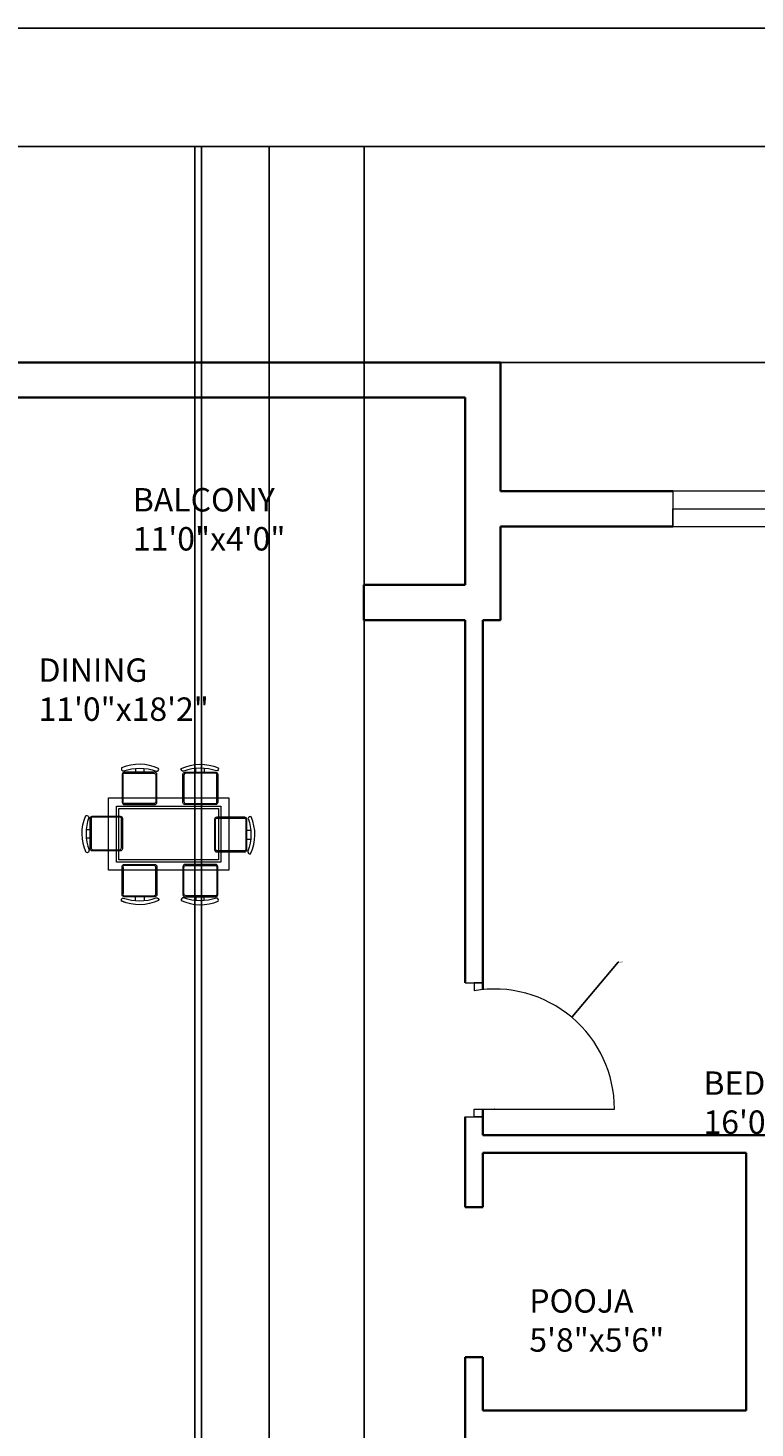
# Model space of a CAD drawing. Units: inches. Extents: x 1902 to 2626, y 1199 to 2408.
# Tile 8 of 9: x 2220 to 2407, y 2049 to 2408. Entities that reach past the tile are written whole.
import ezdxf

# ---------------------------------------------------------------- set-up
doc = ezdxf.new("R2010")
doc.units = ezdxf.units.IN
for name, color, linetype, lineweight in [('A-ANNO-DIMS', 2, 'Continuous', 18), ('A-ANNO-TTLB', 7, 'Continuous', 25), ('A-AREA-IDEN', 7, 'Continuous', 18), ('A-DOOR', 31, 'Continuous', 18), ('A-FURN', 8, 'Continuous', 13), ('A-GLAZ', 181, 'Continuous', 18), ('A-WALL', 7, 'Continuous', 35)]:
    doc.layers.add(name, color=color, linetype=linetype, lineweight=lineweight)
doc.styles.get("Standard").update_dxf_attribs({"font": 'arial.ttf'})
doc.dimstyles.get("Standard").update_dxf_attribs({"dimtxt": 0.18, "dimasz": 0.18, "dimexe": 0.18, "dimexo": 0.0625, "dimgap": 0.09, "dimtad": 0, "dimtih": 1, "dimtoh": 1, "dimdec": 4, "dimzin": 0, "dimdsep": 46, "dimtxsty": 'Standard', "dimcen": 0.09, "dimadec": 0, "dimazin": 0, "dimtfac": 1, "dimtdec": 4, "dimtofl": 0, "dimtmove": 0, "dimatfit": 3, "dimfxl": 1, "dimtolj": 1, "dimtzin": 0, "dimarcsym": 0})

# ---------------------------------------------------------------- blocks, each defined once
blk = doc.blocks.new('WINDOW-60-A')
for p, q in [((0, 9), (0, 0)), ((60, 9), (0, 9)), ((60, 4.5), (60, 9)), ((60, 9), (60, 0)), ((0, 0), (0, 4.5)), ((0, 4.5), (60, 4.5)), ((0, 0), (60, 0))]:
    blk.add_line(p, q)
blk = doc.blocks.new('TABLE-DINING-RECT')
for points in [[(0, 18.51), (30.84, 18.51), (30.84, 0), (0, 0)], [(2.06, 16.45), (28.79, 16.45), (28.79, 2.06), (2.06, 2.06)], [(2.67, 15.83), (28.17, 15.83), (28.17, 2.67), (2.67, 2.67)]]:
    blk.add_lwpolyline(points, close=True)
blk = doc.blocks.new('CHAIR-DINING')
for points in [[(8.55, 2.06), (0.75, 2.06, -0.414214), (0.2, 2.6), (0.2, 9.77, -0.414214), (0.75, 10.32), (8.55, 10.32, -0.414214), (9.09, 9.77), (9.09, 2.6, -0.414214), (8.55, 2.06)], [(8.91, 1.78, -0.578392), (9.54, 1.08, -0.214524), (0.06, 0.96, -0.552014), (0.5, 1.72, 0.175809), (8.91, 1.78)], [(5.81, 2.06), (5.81, 1.07, 0.064759)]]:
    blk.add_lwpolyline(points, format="xyb")
blk.add_lwpolyline([(0.75, 2.3), (8.3, 2.3, 0.414214), (8.85, 2.85), (8.85, 9.53, 0.414214), (8.3, 10.07), (0.75, 10.07, 0.512069), (0.45, 9.53), (0.45, 2.85, 0.512069)], format="xyb", close=True)
blk.add_lwpolyline([(3.63, 1.05), (3.63, 2.06)])
blk = doc.blocks.new('*D28')
at = {"layer": 'A-ANNO-DIMS', "color": 0, "lineweight": -2, "transparency": 16777216}
for p, q in [((1999.35, 2289.54), (1999.35, 2377.95)), ((1999.53, 2377.77), (2268.21, 2377.77)), ((2537.67, 2377.77), (2269, 2377.77)), ((2537.85, 2289.54), (2537.85, 2377.95))]:
    blk.add_line(p, q, dxfattribs=at)
at = {"layer": 'A-ANNO-DIMS', "color": 0, "transparency": 16777216}
for points in [[(1999.53, 2377.8), (1999.53, 2377.74), (1999.35, 2377.77)], [(2537.67, 2377.8), (2537.67, 2377.74), (2537.85, 2377.77)]]:
    blk.add_solid(points, dxfattribs=at)
at = {"layer": 'Defpoints', "color": 0, "transparency": 16777216}
for p in [(2537.85, 2377.77), (1999.35, 2289.47), (2537.85, 2289.47)]:
    blk.add_point(p, dxfattribs=at)
at = {"layer": 'A-ANNO-DIMS', "color": 0, "transparency": 16777216, "insert": (2268.6, 2377.77), "char_height": 0.18, "attachment_point": 5}
blk.add_mtext('\\A1;538.5', dxfattribs=at)
blk = doc.blocks.new('*D35')
at = {"layer": 'A-ANNO-DIMS', "color": 0, "lineweight": -2, "transparency": 16777216}
for p, q in [((2341.41, 2322.47), (2593.33, 2322.47)), ((2593.15, 2322.29), (2593.15, 2306.16)), ((2593.15, 2289.65), (2593.15, 2305.79)), ((2537.91, 2289.47), (2593.33, 2289.47))]:
    blk.add_line(p, q, dxfattribs=at)
at = {"layer": 'A-ANNO-DIMS', "color": 0, "transparency": 16777216}
for points in [[(2593.12, 2322.29), (2593.18, 2322.29), (2593.15, 2322.47)], [(2593.12, 2289.65), (2593.18, 2289.65), (2593.15, 2289.47)]]:
    blk.add_solid(points, dxfattribs=at)
at = {"layer": 'Defpoints', "color": 0, "transparency": 16777216}
for p in [(2341.35, 2322.47), (2593.15, 2322.47), (2537.85, 2289.47)]:
    blk.add_point(p, dxfattribs=at)
at = {"layer": 'A-ANNO-DIMS', "color": 0, "transparency": 16777216, "insert": (2593.15, 2305.97), "char_height": 0.18, "attachment_point": 5}
blk.add_mtext('\\A1;33', dxfattribs=at)
blk = doc.blocks.new('*D41')
at = {"layer": 'A-ANNO-DIMS', "color": 0, "lineweight": -2, "transparency": 16777216}
for p, q in [((2264.77, 1723.47), (2264.77, 2377.95)), ((2264.95, 2377.77), (2285.22, 2377.77)), ((2306.27, 2377.77), (2286.01, 2377.77)), ((2306.45, 1723.47), (2306.45, 2377.95))]:
    blk.add_line(p, q, dxfattribs=at)
at = {"layer": 'A-ANNO-DIMS', "color": 0, "transparency": 16777216}
for points in [[(2264.95, 2377.8), (2264.95, 2377.74), (2264.77, 2377.77)], [(2306.27, 2377.8), (2306.27, 2377.74), (2306.45, 2377.77)]]:
    blk.add_solid(points, dxfattribs=at)
at = {"layer": 'Defpoints', "color": 0, "transparency": 16777216}
for p in [(2306.45, 2377.77), (2264.77, 1723.41), (2306.45, 1723.41)]:
    blk.add_point(p, dxfattribs=at)
at = {"layer": 'A-ANNO-DIMS', "color": 0, "transparency": 16777216, "insert": (2285.61, 2377.77), "char_height": 0.18, "attachment_point": 5}
blk.add_mtext('\\A1;41.68', dxfattribs=at)
blk = doc.blocks.new('*D43')
at = {"layer": 'A-ANNO-DIMS', "color": 0, "lineweight": -2, "transparency": 16777216}
for p, q in [((2263.07, 1800.47), (2263.07, 2377.95)), ((2263.25, 2377.77), (2272.13, 2377.77)), ((2281.92, 2377.77), (2273.04, 2377.77)), ((2282.1, 1800.47), (2282.1, 2377.95))]:
    blk.add_line(p, q, dxfattribs=at)
at = {"layer": 'A-ANNO-DIMS', "color": 0, "transparency": 16777216}
for points in [[(2263.25, 2377.8), (2263.25, 2377.74), (2263.07, 2377.77)], [(2281.92, 2377.8), (2281.92, 2377.74), (2282.1, 2377.77)]]:
    blk.add_solid(points, dxfattribs=at)
at = {"layer": 'Defpoints', "color": 0, "transparency": 16777216}
for p in [(2282.1, 2377.77), (2263.07, 1800.41), (2282.1, 1800.41)]:
    blk.add_point(p, dxfattribs=at)
at = {"layer": 'A-ANNO-DIMS', "color": 0, "transparency": 16777216, "insert": (2272.58, 2377.77), "char_height": 0.18, "attachment_point": 5}
blk.add_mtext('\\A1;19.024', dxfattribs=at)
blk = doc.blocks.new('*D46')
at = {"layer": 'A-ANNO-DIMS', "color": 0, "lineweight": -2, "transparency": 16777216}
for p, q in [((2371.55, 2168.82), (2359.77, 2154.83)), ((2371.73, 2168.82), (2371.55, 2168.82)), ((2339.74, 2131.16), (2339.92, 2131.16)), ((2339.83, 2131.07), (2339.83, 2131.25))]:
    blk.add_line(p, q, dxfattribs=at)
at = {"layer": 'A-ANNO-DIMS', "color": 0, "transparency": 16777216}
blk.add_solid([(2359.75, 2154.85), (2359.79, 2154.81), (2359.65, 2154.7)], dxfattribs=at)
at = {"layer": 'Defpoints', "color": 0, "transparency": 16777216}
for p in [(2359.65, 2154.7), (2339.83, 2131.16)]:
    blk.add_point(p, dxfattribs=at)
at = {"layer": 'A-ANNO-DIMS', "color": 0, "transparency": 16777216, "insert": (2372.28, 2168.82), "char_height": 0.18, "attachment_point": 5}
blk.add_mtext('\\A1;R30.775', dxfattribs=at)

msp = doc.modelspace()

# ---------------------------------------------------------------- linework, layer by layer
at = {"layer": 'A-ANNO-TTLB'}
msp.add_lwpolyline([(1901.6928, 2408.1473), (2626.1646, 2408.1473), (2626.1646, 1206.3103), (1901.6928, 1206.3103)], close=True, dxfattribs=at)
at = {"layer": 'A-DOOR'}
for p, q in [((2332.3507, 2163.4878), (2336.8507, 2163.4878)), ((2336.8507, 2163.4878), (2334.6007, 2163.4878)), ((2334.6007, 2163.4878), (2334.6007, 2161.4878)), ((2334.6007, 2129.1591), (2334.6007, 2131.1591)), ((2334.6007, 2131.1591), (2370.6007, 2131.1591)), ((2332.3507, 2129.1591), (2336.8507, 2129.1591)), ((2336.8507, 2129.1591), (2334.6007, 2129.1591))]:
    msp.add_line(p, q, dxfattribs=at)
msp.add_arc((2339.8252, 2131.1591), 30.7755, 360, 99.774014, dxfattribs=at)
at = {"layer": 'A-FURN'}
for points in [[(2244.7449, 2217.8014, -0.17580919), (2253.1458, 2217.7377, 0.57839206), (2253.7822, 2218.4376, 0.21452438), (2244.2994, 2218.5648, 0.55201397), (2244.7449, 2217.8014, -0.06507904)], [(2244.7449, 2217.801, -0.17580919), (2253.1458, 2217.7374, 0.57839206), (2253.7822, 2218.4372, 0.21452438), (2244.2994, 2218.5645, 0.55201397), (2244.7449, 2217.801, -0.06507904)], [(2252.7893, 2217.4642), (2244.9903, 2217.4642, 0.41421356), (2244.4446, 2216.9186), (2244.4446, 2209.7475, 0.41421356), (2244.9903, 2209.2018), (2252.7893, 2209.2018, 0.41421356), (2253.335, 2209.7475), (2253.335, 2216.9186, 0.41421356), (2252.7893, 2217.4642)], [(2252.7894, 2217.4639), (2244.9903, 2217.4639, 0.41421356), (2244.4447, 2216.9182), (2244.4447, 2209.7471, 0.41421356), (2244.9903, 2209.2015), (2252.7894, 2209.2015, 0.41421356), (2253.335, 2209.7471), (2253.335, 2216.9182, 0.41421356), (2252.7894, 2217.4639)], [(2250.0499, 2217.4642), (2250.0499, 2218.4505, -0.06475861)], [(2250.0499, 2217.4639), (2250.0499, 2218.4502, -0.06475861)], [(2260.2182, 2217.7377, -0.57839206), (2259.5818, 2218.4376, -0.21452438), (2269.0645, 2218.5648, -0.55201397), (2268.619, 2217.8014, 0.1758092), (2260.2182, 2217.7378)], [(2260.2182, 2217.7374, -0.57839206), (2259.5818, 2218.4372, -0.21452438), (2269.0646, 2218.5645, -0.55201397), (2268.6191, 2217.801, 0.1758092), (2260.2182, 2217.7374)], [(2268.3737, 2217.4642, -0.41421356), (2268.9193, 2216.9186), (2268.9193, 2209.7475, -0.41421356), (2268.3737, 2209.2018), (2260.5746, 2209.2018, -0.41421356), (2260.029, 2209.7475), (2260.029, 2216.9186, -0.41421356), (2260.5746, 2217.4642), (2268.3737, 2217.4642)], [(2268.3737, 2217.4639, -0.41421356), (2268.9193, 2216.9182), (2268.9193, 2209.7471, -0.41421356), (2268.3737, 2209.2015), (2260.5746, 2209.2015, -0.41421356), (2260.029, 2209.7471), (2260.029, 2216.9182, -0.41421356), (2260.5746, 2217.4639), (2268.3737, 2217.4639)], [(2263.314, 2217.4642), (2263.314, 2218.4505, 0.06475861)], [(2263.314, 2217.4639), (2263.314, 2218.4502, 0.06475861)], [(2235.956, 2197.5146, -0.57839206), (2235.2562, 2196.8782, -0.21452438), (2235.129, 2206.3609, -0.55201397), (2235.8924, 2205.9154, 0.17580937), (2235.956, 2197.5146)], [(2235.956, 2197.5143, -0.57839206), (2235.2562, 2196.8778, -0.21452438), (2235.129, 2206.3606, -0.55201397), (2235.8924, 2205.9151, 0.17580937), (2235.956, 2197.5143)], [(2236.2296, 2205.6701, -0.41421356), (2236.7752, 2206.2157), (2243.9463, 2206.2157, -0.41421356), (2244.4919, 2205.6701), (2244.4919, 2197.871, -0.41421356), (2243.9463, 2197.3254), (2236.7752, 2197.3254, -0.41421356), (2236.2296, 2197.871), (2236.2296, 2205.6701)], [(2236.2296, 2205.6697, -0.41421356), (2236.7752, 2206.2154), (2243.9463, 2206.2154, -0.41421356), (2244.4919, 2205.6697), (2244.4919, 2197.8707, -0.41421356), (2243.9463, 2197.325), (2236.7752, 2197.325, -0.41421356), (2236.2296, 2197.8707), (2236.2296, 2205.6697)], [(2276.3911, 2205.403, 0.41421356), (2275.8455, 2205.9486), (2268.6744, 2205.9486, 0.41421356), (2268.1287, 2205.403), (2268.1287, 2197.6039, 0.41421356), (2268.6744, 2197.0583), (2275.8455, 2197.0583, 0.41421356), (2276.3911, 2197.6039), (2276.3911, 2205.403)], [(2276.3911, 2205.4026, 0.41421356), (2275.8455, 2205.9483), (2268.6744, 2205.9483, 0.41421356), (2268.1288, 2205.4026), (2268.1288, 2197.6036, 0.41421356), (2268.6744, 2197.0579), (2275.8455, 2197.0579, 0.41421356), (2276.3911, 2197.6036), (2276.3911, 2205.4026)], [(2276.7283, 2205.6483, -0.17580919), (2276.6646, 2197.2475, 0.57839206), (2277.3645, 2196.6111, 0.21452438), (2277.4917, 2206.0938, 0.55201397), (2276.7283, 2205.6483, -0.06507904)], [(2276.7283, 2205.648, -0.17580919), (2276.6647, 2197.2472, 0.57839206), (2277.3645, 2196.6107, 0.21452438), (2277.4917, 2206.0935, 0.55201397), (2276.7283, 2205.648, -0.06507904)], [(2236.2296, 2200.6104), (2235.2432, 2200.6104, 0.06475861)], [(2236.2296, 2200.6101), (2235.2432, 2200.6101, 0.06475861)], [(2276.3911, 2200.3433), (2277.3774, 2200.3433, -0.06475861)], [(2276.3911, 2200.343), (2277.3775, 2200.343, -0.06475861)], [(2252.7893, 2185.5869), (2244.9903, 2185.5869, -0.41421356), (2244.4446, 2186.1326), (2244.4446, 2193.3037, -0.41421356), (2244.9903, 2193.8493), (2252.7893, 2193.8493, -0.41421356), (2253.335, 2193.3037), (2253.335, 2186.1326, -0.41421356), (2252.7893, 2185.5869)], [(2268.3737, 2185.5869, 0.41421356), (2268.9193, 2186.1326), (2268.9193, 2193.3037, 0.41421356), (2268.3737, 2193.8493), (2260.5746, 2193.8493, 0.41421356), (2260.029, 2193.3037), (2260.029, 2186.1326, 0.41421356), (2260.5746, 2185.5869), (2268.3737, 2185.5869)], [(2268.3737, 2185.5866, 0.41421356), (2268.9193, 2186.1322), (2268.9193, 2193.3033, 0.41421356), (2268.3737, 2193.849), (2260.5746, 2193.849, 0.41421356), (2260.029, 2193.3033), (2260.029, 2186.1322, 0.41421356), (2260.5746, 2185.5866), (2268.3737, 2185.5866)], [(2253.1458, 2185.3134, -0.57839206), (2253.7822, 2184.6136, -0.21452438), (2244.2994, 2184.4863, -0.55201397), (2244.7449, 2185.2498, 0.17580929), (2253.1458, 2185.3134)], [(2250.0499, 2185.5869), (2250.0499, 2184.6006, 0.06475861)], [(2268.619, 2185.2498, -0.17580928), (2260.2182, 2185.3134, 0.57839206), (2259.5818, 2184.6136, 0.21452438), (2269.0645, 2184.4863, 0.55201397), (2268.619, 2185.2498, -0.06507904)], [(2268.6191, 2185.2494, -0.17580928), (2260.2182, 2185.3131, 0.57839206), (2259.5818, 2184.6133, 0.21452438), (2269.0646, 2184.486, 0.55201397), (2268.6191, 2185.2494, -0.06507904)], [(2263.314, 2185.5869), (2263.314, 2184.6006, -0.06475861)], [(2263.314, 2185.5866), (2263.314, 2184.6003, -0.06475861)]]:
    msp.add_lwpolyline(points, format="xyb", dxfattribs=at)
for points in [[(2244.9936, 2217.2184), (2252.5435, 2217.2184, -0.41421356), (2253.0892, 2216.6728), (2253.0892, 2209.9933, -0.41421356), (2252.5435, 2209.4477), (2244.9936, 2209.4477, -0.51206948), (2244.6905, 2209.9933), (2244.6905, 2216.6728, -0.51206948)], [(2244.9936, 2217.2181), (2252.5435, 2217.2181, -0.41421356), (2253.0892, 2216.6724), (2253.0892, 2209.993, -0.41421356), (2252.5435, 2209.4473), (2244.9936, 2209.4473, -0.51206948), (2244.6905, 2209.993), (2244.6905, 2216.6724, -0.51206948)], [(2268.3704, 2217.2184), (2260.8204, 2217.2184, 0.41421356), (2260.2748, 2216.6728), (2260.2748, 2209.9933, 0.41421356), (2260.8204, 2209.4477), (2268.3704, 2209.4477, 0.51206948), (2268.6735, 2209.9933), (2268.6735, 2216.6728, 0.51206948)], [(2268.3704, 2217.2181), (2260.8204, 2217.2181, 0.41421356), (2260.2748, 2216.6724), (2260.2748, 2209.993, 0.41421356), (2260.8204, 2209.4473), (2268.3704, 2209.4473, 0.51206948), (2268.6735, 2209.993), (2268.6735, 2216.6724, 0.51206948)], [(2236.4754, 2205.6668), (2236.4754, 2198.1168, 0.41421356), (2237.021, 2197.5712), (2243.7005, 2197.5712, 0.41421356), (2244.2461, 2198.1168), (2244.2461, 2205.6668, 0.51206948), (2243.7005, 2205.9699), (2237.021, 2205.9699, 0.51206948)], [(2236.4754, 2205.6664), (2236.4754, 2198.1165, 0.41421356), (2237.021, 2197.5709), (2243.7005, 2197.5709, 0.41421356), (2244.2461, 2198.1165), (2244.2461, 2205.6664, 0.51206948), (2243.7005, 2205.9696), (2237.021, 2205.9696, 0.51206948)], [(2276.1453, 2205.3997), (2276.1453, 2197.8497, -0.41421356), (2275.5997, 2197.3041), (2268.9202, 2197.3041, -0.41421356), (2268.3746, 2197.8497), (2268.3746, 2205.3997, -0.51206948), (2268.9202, 2205.7028), (2275.5997, 2205.7028, -0.51206948)], [(2276.1453, 2205.3993), (2276.1453, 2197.8494, -0.41421356), (2275.5997, 2197.3038), (2268.9202, 2197.3038, -0.41421356), (2268.3746, 2197.8494), (2268.3746, 2205.3993, -0.51206948), (2268.9202, 2205.7025), (2275.5997, 2205.7025, -0.51206948)], [(2244.9936, 2185.8327), (2252.5435, 2185.8327, 0.41421356), (2253.0892, 2186.3784), (2253.0892, 2193.0579, 0.41421356), (2252.5435, 2193.6035), (2244.9936, 2193.6035, 0.51206948), (2244.6905, 2193.0579), (2244.6905, 2186.3784, 0.51206948)], [(2268.3704, 2185.8327), (2260.8204, 2185.8327, -0.41421356), (2260.2748, 2186.3784), (2260.2748, 2193.0579, -0.41421356), (2260.8204, 2193.6035), (2268.3704, 2193.6035, -0.51206948), (2268.6735, 2193.0579), (2268.6735, 2186.3784, -0.51206948)], [(2268.3704, 2185.8324), (2260.8204, 2185.8324, -0.41421356), (2260.2748, 2186.3781), (2260.2748, 2193.0575, -0.41421356), (2260.8204, 2193.6032), (2268.3704, 2193.6032, -0.51206948), (2268.6735, 2193.0575), (2268.6735, 2186.3781, -0.51206948)]]:
    msp.add_lwpolyline(points, format="xyb", close=True, dxfattribs=at)
for points in [[(2247.8668, 2218.4685), (2247.8668, 2217.4642)], [(2247.8669, 2218.4681), (2247.8669, 2217.4639)], [(2265.4971, 2218.4685), (2265.4971, 2217.4642)], [(2265.4971, 2218.4681), (2265.4971, 2217.4639)], [(2235.2253, 2202.7935), (2236.2296, 2202.7935)], [(2235.2253, 2202.7932), (2236.2296, 2202.7932)], [(2277.3954, 2202.5264), (2276.3911, 2202.5264)], [(2277.3954, 2202.5261), (2276.3911, 2202.5261)], [(2247.8668, 2184.5827), (2247.8668, 2185.5869)], [(2265.4971, 2184.5827), (2265.4971, 2185.5869)], [(2265.4971, 2184.5823), (2265.4971, 2185.5866)]]:
    msp.add_lwpolyline(points, dxfattribs=at)
at = {"layer": 'A-WALL'}
for p, q in [((2341.3507, 2322.4733), (2191.3507, 2322.4733)), ((2341.3507, 2313.4733), (2341.3507, 2322.4733)), ((2200.3507, 2313.4733), (2332.3507, 2313.4733)), ((2332.3507, 2313.4733), (2332.3507, 2280.4733)), ((2341.3507, 2289.4733), (2341.3507, 2313.4733)), ((2341.3507, 2289.4733), (2385.516, 2289.4733)), ((2332.3507, 2280.4733), (2332.3507, 2265.4733)), ((2341.3507, 2280.4733), (2385.516, 2280.4733)), ((2341.3507, 2256.4733), (2341.3507, 2280.4733)), ((2306.3713, 2265.4733), (2306.3713, 2256.4733)), ((2306.3713, 2265.4733), (2332.3507, 2265.4733)), ((2306.3713, 2256.4733), (2332.3507, 2256.4733)), ((2332.3507, 2256.4733), (2332.3507, 2256.4733)), ((2332.3507, 2256.4733), (2332.3507, 2163.4878)), ((2336.8507, 2256.4733), (2341.3507, 2256.4733)), ((2336.8507, 2256.4733), (2336.8507, 2161.7905)), ((2336.8507, 2131.1591), (2336.8507, 2124.4733)), ((2332.3507, 2129.1591), (2332.3507, 2118.0201)), ((2336.8507, 2124.4733), (2464.8563, 2124.4733)), ((2336.8507, 2119.9733), (2404.3507, 2119.9733)), ((2336.8507, 2106.0811), (2336.8507, 2119.9733)), ((2404.3507, 2119.9733), (2404.3507, 2053.9733)), ((2332.3507, 2118.0201), (2332.3507, 2106.0811)), ((2332.3507, 2106.0811), (2336.8507, 2106.0811)), ((2332.3507, 2067.5809), (2332.3507, 2044.9733)), ((2332.3507, 2067.5809), (2336.8507, 2067.5809)), ((2336.8507, 2053.9733), (2336.8507, 2067.5809)), ((2336.8507, 2053.9733), (2404.3507, 2053.9733))]:
    msp.add_line(p, q, dxfattribs=at)

# ---------------------------------------------------------------- block references
at = {"layer": 'A-FURN'}
for name, p in [('TABLE-DINING-RECT', (2240.93, 2192.37)), ('TABLE-DINING-RECT', (2240.93, 2192.3697)), ('CHAIR-DINING', (2244.24, 2183.53))]:
    msp.add_blockref(name, p, dxfattribs=at)
at = {"layer": 'A-GLAZ'}
msp.add_blockref('WINDOW-60-A', (2385.52, 2280.47), dxfattribs=at)

# ---------------------------------------------------------------- texts
at = {"layer": 'A-AREA-IDEN', "char_height": 6, "attachment_point": 1}
for s, width, insert in [('BALCONY\\P11\'0"x4\'0"', 152.57794, (2247.1836, 2290.2825)), ('DINING\\P11\'0"x18\'2"', 158.944551, (2223.0177, 2246.6393)), ('BEDROOM\\P16\'0"x13\'0"', 174.865201, (2393.4079, 2140.8318)), ('POOJA\\P5\'8"x5\'6"', 93.004151, (2348.7747, 2085.0333))]:
    msp.add_mtext_dynamic_manual_height_columns(s, width=width, gutter_width=12.5, heights=[0], dxfattribs=dict(at, insert=insert))

# ---------------------------------------------------------------- dimensions: what is measured, and where the dimension line sits
at = {"layer": 'A-ANNO-DIMS'}
for base, p1, p2, override, picture, middle in [((2537.8507, 2377.7733), (1999.3507, 2289.4733), (2537.8507, 2289.4733), {"dimdec": 1, "dimlfac": 1, "dimrnd": 0, "dimzin": 0, "dimdsep": 46, "dimlunit": 2}, '*D28', (2268.6007, 2377.7733)), ((2282.0954, 2377.7733), (2263.071, 1800.4076), (2282.0954, 1800.4076), {"dimdec": 3, "dimlfac": 1, "dimrnd": 0, "dimzin": 0, "dimdsep": 46, "dimlunit": 2}, '*D43', (2272.5832, 2377.7733)), ((2306.4528, 2377.7733), (2264.7741, 1723.4115), (2306.4528, 1723.4115), {"dimdec": 2, "dimlfac": 1, "dimrnd": 0, "dimzin": 0, "dimdsep": 46, "dimlunit": 2}, '*D41', (2285.6134, 2377.7733))]:
    dim = msp.add_linear_dim(base=base, p1=p1, p2=p2, dimstyle='Standard', override=override, dxfattribs=at)
    dim.commit()
    dim.dimension.update_dxf_attribs({"geometry": picture, "text_midpoint": middle})
dim = msp.add_linear_dim(base=(2593.1507, 2322.4733), p1=(2537.8507, 2289.4733), p2=(2341.3507, 2322.4733), angle=90, dimstyle='Standard', override={"dimdec": 0, "dimlfac": 1, "dimrnd": 0, "dimzin": 0, "dimdsep": 46, "dimlunit": 2}, dxfattribs=at)
dim.commit()
dim.dimension.update_dxf_attribs({"geometry": '*D35', "text_midpoint": (2593.1507, 2305.9733)})
dim = msp.add_radius_dim(center=(2339.8252, 2131.1591), mpoint=(2359.6541, 2154.6951), dimstyle='Standard', override={"dimdec": 3, "dimlfac": 1, "dimrnd": 0, "dimzin": 0, "dimdsep": 46, "dimlunit": 2}, dxfattribs=at)
dim.commit()
dim.dimension.update_dxf_attribs({"geometry": '*D46', "text_midpoint": (2372.2819, 2168.8167), "dimtype": 164})

doc.saveas('drawing.dxf')
